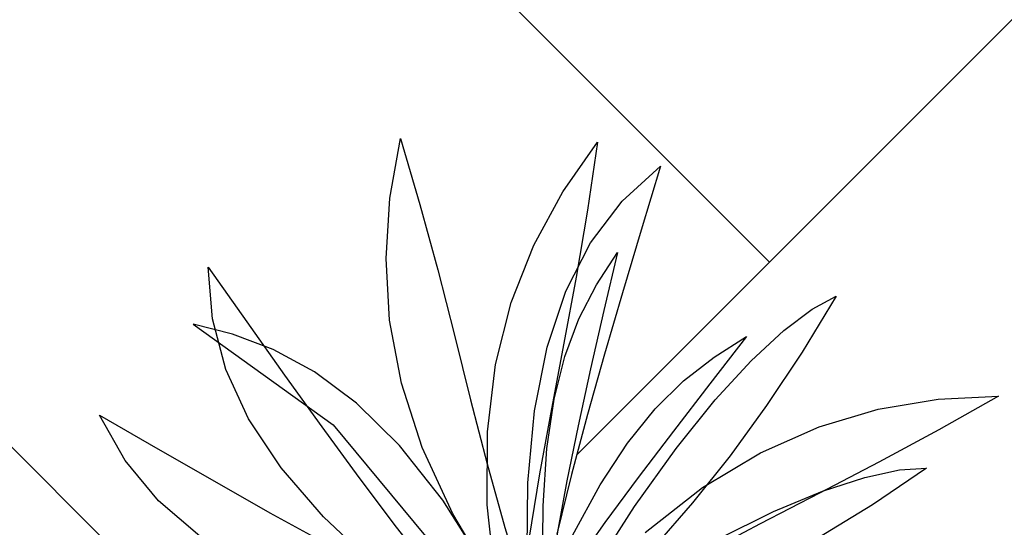
# Model space of a CAD drawing. Units: inches. Extents: x 3590 to 5167, y 65 to 1917.
# Tile 41 of 100: x 5035 to 5065, y 1357 to 1372. Entities that reach past the tile are written whole.
import ezdxf

# ---------------------------------------------------------------- set-up
doc = ezdxf.new("R2010")
doc.units = ezdxf.units.IN
doc.layers.add('A-FLOR-PATT', color=8, linetype='Continuous', lineweight=13)
doc.layers.add('L-PLNT', color=94, linetype='Continuous', lineweight=18)
doc.layers.add('DIENHOA', color=3, linetype='Continuous')

# ---------------------------------------------------------------- blocks, each defined once
blk = doc.blocks.new('Cay03_mb')
at = {"layer": 'DIENHOA'}
for p, q in [((118.6, 555.3), (166.2, 599.1)), ((166.2, 599.1), (142.2, 519.4)), ((79.5, 503.7), (118.6, 555.3)), ((142.2, 519.4), (119, 441.7)), ((48.6, 443.6), (79.5, 503.7)), ((25.5, 374.3), (48.6, 443.6)), ((119, 441.7), (96.7, 365.6)), ((-365.2, 390.3), (-414.4, 402.8)), ((-414.4, 402.8), (-240.2, 277.8)), ((-314.9, 371.3), (-365.2, 390.3)), ((-263.5, 343.5), (-314.9, 371.3)), ((9.9, 295.3), (25.5, 374.3)), ((96.7, 365.6), (75.6, 290.6)), ((-211.2, 304.6), (-263.5, 343.5)), ((436.8, 297.2), (511, 309.6)), ((511, 309.6), (585.9, 313.5)), ((585.9, 313.5), (511.8, 271.4)), ((-158, 252.3), (-211.2, 304.6)), ((1.6, 205.7), (9.9, 295.3)), ((363.4, 275.4), (436.8, 297.2)), ((75.6, 290.6), (55.7, 216.3)), ((-240.2, 277.8), (-88.4, 94.9)), ((290.6, 243.2), (363.4, 275.4)), ((511.8, 271.4), (437.6, 231.5)), ((-104.2, 184.4), (-158, 252.3)), ((218.5, 199.8), (290.6, 243.2)), ((437.6, 231.5), (363.7, 192.9)), ((55.7, 216.3), (37.3, 142.1)), ((0.2, 104.9), (1.6, 205.7)), ((147, 144.1), (218.5, 199.8)), ((-49.6, 98.5), (-104.2, 184.4)), ((363.7, 192.9), (290.2, 154.9)), ((290.2, 154.9), (217.4, 116.6))]:
    blk.add_line(p, q, dxfattribs=at)
for points in [[(23.7, -5.4), (-41, 82.2), (-91.8, 167.1), (-129.7, 249.5), (-155.6, 329.6), (-170.2, 407.8), (-174.7, 484.2), (-169.8, 559.3), (-156.5, 633.1)], [(-156.5, 633.1), (-132.5, 551.3), (-110.5, 470), (-89.8, 389.2), (-69.6, 309), (-49, 229.4), (-27.1, 150.4), (-3.2, 72.1), (23.7, -5.4)], [(-16.4, -26.7), (-38.3, 80), (-48.9, 178.3), (-48.7, 269), (-38.5, 352.6), (-19.1, 429.7), (9, 501), (44.9, 567.1), (87.9, 628.5)], [(87.9, 628.5), (75.5, 544.2), (61.3, 461.2), (46.1, 379.1), (30.8, 297.8), (16.1, 216.9), (2.9, 136), (-8.3, 54.9), (-16.4, -26.7)], [(23.7, -5.4), (19.8, 93), (20.3, 177), (25, 248.5), (34, 309.8), (47.3, 362.7), (64.9, 409.3), (86.8, 451.7), (112.9, 491.9)], [(112.9, 491.9), (96, 419.7), (79.5, 347.4), (63.9, 276.5), (50, 208.4), (38.4, 144.8), (29.7, 86.9), (24.6, 36.3), (23.7, -5.4)], [(-395.6, 473.7), (-347.5, 405.6), (-300.6, 339.5), (-254.3, 275.1), (-208.3, 212.3), (-161.9, 150.9), (-114.8, 90.7), (-66.5, 31.6), (-16.4, -26.7)], [(-16.4, -26.7), (-108.3, 38.6), (-186.9, 101.7), (-252.4, 163.5), (-305.1, 224.4), (-345.4, 285.2), (-373.7, 346.6), (-390.4, 409.2), (-395.6, 473.7)], [(384.3, 437.5), (342.2, 367.8), (298.1, 301.7), (252.6, 239.4), (206.1, 181.1), (159.4, 127.2), (113, 78), (67.6, 33.6), (23.7, -5.4)], [(23.7, -5.4), (79.9, 91.7), (134.1, 176.2), (185.8, 248.4), (234.3, 308.7), (279, 357.3), (319.3, 394.8), (354.6, 421.4), (384.3, 437.5)], [(273.2, 387.3), (227.6, 328.8), (182.3, 270.1), (138.4, 212.3), (97.2, 156.4), (60, 103.4), (27.8, 54.6), (1.9, 10.8), (-16.4, -26.7)], [(-16.4, -26.7), (21.4, 64.2), (57, 140.3), (91.4, 203.3), (125.2, 255.1), (159.5, 297.5), (195, 332.5), (232.7, 361.8), (273.2, 387.3)], [(-530.5, 289.7), (-458.3, 248.1), (-387.9, 207.8), (-318.9, 168.7), (-250.8, 131.1), (-182.9, 94.8), (-114.9, 59.9), (-46.2, 26.5), (23.7, -5.4)], [(23.7, -5.4), (-87.2, 15.2), (-185, 39.6), (-270.3, 68.2), (-343.7, 101.4), (-405.9, 139.7), (-457.3, 183.5), (-498.7, 233.4), (-530.5, 289.7)], [(496.7, 224), (429.4, 178.4), (361.6, 136.9), (294.1, 99.5), (227.5, 66.1), (162.4, 36.7), (99.7, 11.5), (39.8, -9.7), (-16.4, -26.7)], [(-16.4, -26.7), (75.4, 37.9), (160.1, 91.8), (237.3, 135.7), (306.6, 170), (367.6, 195.4), (419.9, 212.5), (463.1, 221.9), (496.7, 224)]]:
    blk.add_lwpolyline(points, dxfattribs=at)

msp = doc.modelspace()

# ---------------------------------------------------------------- hatches: boundary and pattern name
at = {"layer": 'A-FLOR-PATT', "transparency": 33554687}
h = msp.add_hatch(dxfattribs=at)
h.set_pattern_fill('AR-HBONE', color=256, scale=0.2)
h.set_pattern_definition([(45, (-588.972, 0), (0, 28.73682), [60.96, -20.32]), (135, (-574.604, 14.368), (3e-15, 28.73682), [60.96, -20.32])])
h.paths.add_polyline_path([(5071.274, 1796.999), (4933.274, 1796.999), (4933.274, 1753.999), (4962.774, 1753.999, -0.414214), (4928.774, 1719.999), (4933.274, 1718.999), (4933.274, 1334.999), (5071.274, 1334.999)])
h.paths.add_polyline_path([(4951.78, 1521.077), (4951.715, 1521.04), (4951.563, 1520.895)], flags=16)
h.paths.add_polyline_path([(4952.267, 1521.376), (4952.198, 1521.371), (4952.198, 1521.356)], flags=0)
h.paths.add_polyline_path([(4967.051, 1529.728), (4965.231, 1528.694), (4963.411, 1527.714), (4961.756, 1526.851), (4963.589, 1527.449), (4964.036, 1527.478), (4962.975, 1527.249), (4961.76, 1526.852), (4959.792, 1525.834), (4958.005, 1524.895), (4956.24, 1523.93), (4954.504, 1522.919), (4954.129, 1522.682), (4953.361, 1521.997), (4953.366, 1521.998), (4953.605, 1522.064), (4955.106, 1522.761), (4956.921, 1523.434), (4958.678, 1523.915), (4960.358, 1524.2), (4961.945, 1524.286), (4964.171, 1524.108), (4965.958, 1523.309), (4963.863, 1522.976), (4965.187, 1522.499), (4963.366, 1522.497), (4961.545, 1522.487), (4959.764, 1522.461), (4958.304, 1522.419), (4957.974, 1522.388), (4956.307, 1522.232), (4954.718, 1522.071), (4953.251, 1521.899), (4953.525, 1521.623), (4954.331, 1521.379), (4956.243, 1521.23), (4958.039, 1520.93), (4959.684, 1520.483), (4961.16, 1519.896), (4963.107, 1518.8), (4964.393, 1517.325), (4962.973, 1517.726), (4964.558, 1516.661), (4965.407, 1515.708), (4963.507, 1516.322), (4961.68, 1517.005), (4959.935, 1517.745), (4958.282, 1518.528), (4956.732, 1519.343), (4955.295, 1520.175), (4954.672, 1520.572), (4954.513, 1520.627), (4955.658, 1519.318), (4956.703, 1517.982), (4957.644, 1516.647), (4958.485, 1515.334), (4959.55, 1513.524), (4960.438, 1511.769), (4958.841, 1513.62), (4957.452, 1515.325), (4955.819, 1517.459), (4956.665, 1515.448), (4957.111, 1513.923), (4957.447, 1511.714), (4957.076, 1509.793), (4956.538, 1511.11), (4955.992, 1512.569), (4955.444, 1514.125), (4954.898, 1515.735), (4954.357, 1517.356), (4953.824, 1518.943), (4953.305, 1520.452), (4953.065, 1521.116), (4952.971, 1521.146), (4952.949, 1521.086), (4952.73, 1520.199), (4953.37, 1518.024), (4953.757, 1516.373), (4954.051, 1514.765), (4954.264, 1513.221), (4954.471, 1511.131), (4954.497, 1510.402), (4954.409, 1511.76), (4954.264, 1513.221), (4954.051, 1514.765), (4953.757, 1516.373), (4953.37, 1518.024), (4952.877, 1519.698), (4952.716, 1520.141), (4952.533, 1519.059), (4952.374, 1517.789), (4952.219, 1516.312), (4952.046, 1514.6), (4951.833, 1512.626), (4951.557, 1510.363), (4951.203, 1512.168), (4950.852, 1514.339), (4950.985, 1516.376), (4951.66, 1518.286), (4952.593, 1520.481), (4952.357, 1521.13), (4951.855, 1520.328), (4950.839, 1518.908), (4949.777, 1517.587), (4948.916, 1516.617), (4948.111, 1515.256), (4947.089, 1513.554), (4945.889, 1511.615), (4946.326, 1513.402), (4946.562, 1514.249), (4945.528, 1513.327), (4944.581, 1512.531), (4946.018, 1514.508), (4947.204, 1516.048), (4947.893, 1517.313), (4949.307, 1518.764), (4950.414, 1519.767), (4950.451, 1519.806), (4952.267, 1521.376), (4951.645, 1521.493), (4950.404, 1521.18), (4948.044, 1520.359), (4946.119, 1519.452), (4944.572, 1518.475), (4943.35, 1517.443), (4941.997, 1515.92), (4941.661, 1515.275), (4942.813, 1516.99), (4944.572, 1518.475), (4946.119, 1519.452), (4948.044, 1520.359), (4950.404, 1521.18), (4951.645, 1521.493), (4949.647, 1521.868), (4948.6, 1521.756), (4947.126, 1521.57), (4945.42, 1521.348), (4943.45, 1521.105), (4941.183, 1520.856), (4942.86, 1521.613), (4943.873, 1522.03), (4942.952, 1521.909), (4941.41, 1521.485), (4939.543, 1520.67), (4938.968, 1520.226), (4940.733, 1521.299), (4942.952, 1521.909), (4943.702, 1522.008), (4945.894, 1522.7), (4947.565, 1522.714), (4948.921, 1522.566), (4951.131, 1522.183), (4950.971, 1522.297), (4948.129, 1523.006), (4946.035, 1523.707), (4944.232, 1524.521), (4942.707, 1525.461), (4941.444, 1526.537), (4940.43, 1527.761), (4939.649, 1529.143), (4941.421, 1528.122), (4943.147, 1527.132), (4944.841, 1526.175), (4946.514, 1525.25), (4948.179, 1524.359), (4948.365, 1524.263), (4946.475, 1526.045), (4945.181, 1527.54), (4944.19, 1529.033), (4943.496, 1530.54), (4943.278, 1531.36), (4942.498, 1531.919), (4943.114, 1531.762), (4942.959, 1533.659), (4944.14, 1531.989), (4944.612, 1531.323), (4946.202, 1530.463), (4947.486, 1529.509), (4948.79, 1528.226), (4950.368, 1526.237), (4949.485, 1528.155), (4948.851, 1530.123), (4948.491, 1532.041), (4948.381, 1533.918), (4948.501, 1535.76), (4948.827, 1537.573), (4949.418, 1535.565), (4949.957, 1533.569), (4950.464, 1531.586), (4950.961, 1529.617), (4951.391, 1527.954), (4951.724, 1530.687), (4952.201, 1532.58), (4952.889, 1534.33), (4953.77, 1535.951), (4954.827, 1537.46), (4954.521, 1535.39), (4954.273, 1533.937), (4955.58, 1535.663), (4956.748, 1536.739), (4956.159, 1534.78), (4955.589, 1532.873), (4955.043, 1531.006), (4954.525, 1529.166), (4954.038, 1527.341), (4953.638, 1525.733), (4953.611, 1525.586), (4953.398, 1524.166), (4953.382, 1524.009), (4954.07, 1525.476), (4954.912, 1527.022), (4956.136, 1528.894), (4957.847, 1530.577), (4959.376, 1531.54), (4958.256, 1530.104), (4957.143, 1528.663), (4956.066, 1527.243), (4955.056, 1525.871), (4954.141, 1524.571), (4953.352, 1523.372), (4953.311, 1523.303), (4953.273, 1522.925), (4953.261, 1522.382), (4954.103, 1523.373), (4954.63, 1524.284), (4955.961, 1526.358), (4957.23, 1528.13), (4958.421, 1529.609), (4960.037, 1531.368), (4961.374, 1532.375), (4962.101, 1532.77), (4961.07, 1531.061), (4959.987, 1529.438), (4958.869, 1527.908), (4958.15, 1527.007), (4959.803, 1528.003), (4961.589, 1528.793), (4963.391, 1529.328), (4965.211, 1529.632)], flags=16)
h.paths.add_polyline_path([(4962.944, 1523.182), (4961.107, 1523.422), (4960.392, 1523.362), (4962.35, 1523.331)], flags=0)
h.paths.add_polyline_path([(5049.541, 1584.551), (5049.476, 1584.515), (5049.325, 1584.37)], flags=16)
h.paths.add_polyline_path([(5050.028, 1584.851), (5049.959, 1584.845), (5049.959, 1584.83)], flags=0)
h.paths.add_polyline_path([(5042.333, 1581.949), (5043.88, 1582.926), (5045.806, 1583.833), (5048.165, 1584.654), (5049.406, 1584.967), (5047.408, 1585.342), (5046.361, 1585.231), (5044.888, 1585.044), (5043.181, 1584.822), (5041.211, 1584.579), (5038.944, 1584.33), (5040.622, 1585.087), (5041.634, 1585.504), (5040.713, 1585.383), (5039.171, 1584.959), (5037.304, 1584.144), (5036.729, 1583.7), (5038.494, 1584.773), (5040.713, 1585.383), (5041.463, 1585.482), (5043.655, 1586.174), (5045.326, 1586.188), (5046.682, 1586.04), (5048.893, 1585.657), (5048.732, 1585.771), (5045.891, 1586.48), (5043.796, 1587.181), (5041.994, 1587.996), (5040.468, 1588.935), (5039.205, 1590.011), (5038.191, 1591.235), (5037.41, 1592.617), (5039.182, 1591.596), (5040.909, 1590.607), (5042.602, 1589.649), (5044.275, 1588.724), (5045.94, 1587.833), (5046.126, 1587.738), (5044.237, 1589.519), (5042.942, 1591.015), (5041.952, 1592.508), (5041.257, 1594.014), (5041.039, 1594.834), (5040.26, 1595.393), (5040.875, 1595.237), (5040.721, 1597.133), (5041.901, 1595.463), (5042.373, 1594.798), (5043.963, 1593.938), (5045.247, 1592.983), (5046.552, 1591.701), (5048.129, 1589.712), (5047.247, 1591.63), (5046.613, 1593.597), (5046.252, 1595.515), (5046.142, 1597.392), (5046.262, 1599.234), (5046.588, 1601.047), (5047.179, 1599.039), (5047.718, 1597.043), (5048.225, 1595.06), (5048.722, 1593.091), (5049.152, 1591.429), (5049.485, 1594.161), (5049.962, 1596.054), (5050.65, 1597.804), (5051.532, 1599.425), (5052.589, 1600.934), (5052.283, 1598.864), (5052.034, 1597.411), (5053.341, 1599.137), (5054.509, 1600.213), (5053.92, 1598.254), (5053.35, 1596.348), (5052.805, 1594.48), (5052.286, 1592.64), (5051.799, 1590.815), (5051.4, 1589.207), (5051.373, 1589.06), (5051.159, 1587.64), (5051.143, 1587.483), (5051.831, 1588.95), (5052.673, 1590.496), (5053.898, 1592.368), (5055.608, 1594.051), (5057.137, 1595.014), (5056.017, 1593.578), (5054.904, 1592.137), (5053.828, 1590.717), (5052.817, 1589.345), (5051.902, 1588.046), (5051.113, 1586.846), (5051.072, 1586.777), (5051.034, 1586.399), (5051.022, 1585.856), (5051.864, 1586.847), (5052.391, 1587.758), (5053.723, 1589.832), (5054.991, 1591.604), (5056.182, 1593.083), (5057.798, 1594.842), (5059.135, 1595.849), (5059.863, 1596.244), (5058.831, 1594.535), (5057.749, 1592.912), (5056.63, 1591.382), (5055.912, 1590.482), (5057.564, 1591.477), (5059.35, 1592.267), (5061.152, 1592.802), (5062.972, 1593.106), (5064.812, 1593.203), (5062.992, 1592.169), (5061.172, 1591.188), (5059.518, 1590.325), (5061.35, 1590.924), (5061.797, 1590.952), (5060.737, 1590.723), (5059.521, 1590.326), (5057.553, 1589.308), (5055.766, 1588.369), (5054.002, 1587.404), (5052.265, 1586.393), (5051.891, 1586.156), (5051.122, 1585.471), (5051.127, 1585.472), (5051.366, 1585.538), (5052.867, 1586.235), (5054.682, 1586.908), (5056.439, 1587.389), (5058.12, 1587.675), (5059.706, 1587.76), (5061.933, 1587.583), (5063.719, 1586.783), (5061.624, 1586.45), (5062.949, 1585.973), (5061.127, 1585.971), (5059.307, 1585.961), (5057.525, 1585.935), (5056.065, 1585.893), (5055.735, 1585.862), (5054.068, 1585.707), (5052.479, 1585.546), (5051.012, 1585.373), (5051.286, 1585.097), (5052.092, 1584.853), (5054.004, 1584.704), (5055.8, 1584.404), (5057.446, 1583.958), (5058.921, 1583.37), (5060.868, 1582.274), (5062.154, 1580.799), (5060.734, 1581.2), (5062.32, 1580.135), (5063.168, 1579.182), (5061.269, 1579.796), (5059.441, 1580.479), (5057.696, 1581.219), (5056.043, 1582.003), (5054.493, 1582.817), (5053.057, 1583.649), (5052.433, 1584.047), (5052.274, 1584.101), (5053.42, 1582.793), (5054.464, 1581.457), (5055.405, 1580.121), (5056.247, 1578.809), (5057.311, 1576.998), (5058.199, 1575.244), (5056.602, 1577.094), (5055.213, 1578.799), (5053.58, 1580.933), (5054.427, 1578.922), (5054.872, 1577.397), (5055.208, 1575.189), (5054.838, 1573.267), (5054.299, 1574.584), (5053.754, 1576.043), (5053.206, 1577.599), (5052.659, 1579.209), (5052.118, 1580.83), (5051.585, 1582.417), (5051.066, 1583.927), (5050.826, 1584.59), (5050.733, 1584.62), (5050.711, 1584.561), (5050.491, 1583.673), (5051.131, 1581.498), (5051.518, 1579.847), (5051.813, 1578.24), (5052.026, 1576.695), (5052.233, 1574.605), (5052.258, 1573.876), (5052.17, 1575.234), (5052.026, 1576.695), (5051.813, 1578.24), (5051.518, 1579.847), (5051.131, 1581.498), (5050.638, 1583.172), (5050.477, 1583.615), (5050.294, 1582.533), (5050.136, 1581.263), (5049.981, 1579.786), (5049.807, 1578.074), (5049.594, 1576.1), (5049.318, 1573.837), (5048.965, 1575.642), (5048.613, 1577.813), (5048.747, 1579.85), (5049.421, 1581.76), (5050.354, 1583.955), (5050.118, 1584.604), (5049.616, 1583.802), (5048.6, 1582.382), (5047.538, 1581.061), (5046.677, 1580.091), (5045.872, 1578.73), (5044.85, 1577.028), (5043.651, 1575.089), (5044.087, 1576.877), (5044.324, 1577.723), (5043.289, 1576.801), (5042.342, 1576.005), (5043.779, 1577.982), (5044.966, 1579.522), (5045.655, 1580.787), (5047.068, 1582.239), (5048.175, 1583.241), (5048.213, 1583.28), (5050.028, 1584.851), (5049.406, 1584.967), (5048.165, 1584.654), (5045.806, 1583.833), (5043.88, 1582.926), (5042.333, 1581.949), (5041.111, 1580.917), (5039.758, 1579.394), (5039.423, 1578.749), (5040.575, 1580.464)], flags=16)
h.paths.add_polyline_path([(4954.799, 1533.12), (4954.262, 1532.079), (4953.831, 1530.935), (4953.505, 1529.636), (4953.283, 1528.133), (4953.167, 1526.376), (4953.156, 1524.315), (4953.277, 1521.236), (4952.802, 1521.842), (4951.557, 1521.998), (4950.976, 1521.961), (4952.661, 1521.941), (4952.802, 1521.842), (4953.152, 1523.593), (4953.167, 1526.376), (4953.283, 1528.133), (4953.609, 1530.346), (4954.456, 1532.592)], flags=0)
h.paths.add_polyline_path([(5050.563, 1585.316), (5049.318, 1585.472), (5048.737, 1585.435), (5050.422, 1585.415), (5050.563, 1585.316), (5050.914, 1587.067), (5050.928, 1589.851), (5051.045, 1591.607), (5051.371, 1593.82), (5052.217, 1596.066), (5052.56, 1596.594), (5052.024, 1595.554), (5051.592, 1594.409), (5051.266, 1593.11), (5051.045, 1591.607), (5050.928, 1589.851), (5050.918, 1587.789), (5051.038, 1584.71)], flags=0)
h.paths.add_polyline_path([(5058.153, 1586.836), (5060.111, 1586.805), (5060.705, 1586.656), (5058.868, 1586.896)], flags=0)
h.paths.add_polyline_path([(5049.541, 1430.936), (5049.476, 1430.9), (5049.325, 1430.755)], flags=16)
h.paths.add_polyline_path([(5050.028, 1431.236), (5049.959, 1431.231), (5049.959, 1431.215)], flags=0)
h.paths.add_polyline_path([(5046.588, 1447.432), (5047.179, 1445.425), (5047.718, 1443.429), (5048.225, 1441.446), (5048.722, 1439.476), (5049.152, 1437.814), (5049.485, 1440.546), (5049.962, 1442.439), (5050.65, 1444.189), (5051.532, 1445.811), (5052.589, 1447.319), (5052.283, 1445.249), (5052.034, 1443.796), (5053.341, 1445.522), (5054.509, 1446.598), (5053.92, 1444.64), (5053.35, 1442.733), (5052.805, 1440.865), (5052.286, 1439.025), (5051.799, 1437.201), (5051.4, 1435.592), (5051.373, 1435.445), (5051.159, 1434.025), (5051.143, 1433.868), (5051.831, 1435.335), (5052.673, 1436.881), (5053.898, 1438.753), (5055.608, 1440.436), (5057.137, 1441.4), (5056.017, 1439.963), (5054.904, 1438.522), (5053.828, 1437.102), (5052.817, 1435.73), (5051.902, 1434.431), (5051.113, 1433.231), (5051.072, 1433.162), (5051.034, 1432.784), (5051.022, 1432.242), (5051.864, 1433.232), (5052.391, 1434.143), (5053.723, 1436.217), (5054.991, 1437.989), (5056.182, 1439.468), (5057.798, 1441.227), (5059.135, 1442.235), (5059.863, 1442.629), (5058.831, 1440.921), (5057.749, 1439.298), (5056.63, 1437.767), (5055.912, 1436.867), (5057.564, 1437.863), (5059.35, 1438.652), (5061.152, 1439.187), (5062.972, 1439.491), (5064.812, 1439.588), (5062.992, 1438.554), (5061.172, 1437.573), (5059.518, 1436.71), (5061.35, 1437.309), (5061.797, 1437.337), (5060.737, 1437.108), (5059.521, 1436.711), (5057.553, 1435.693), (5055.766, 1434.754), (5054.002, 1433.789), (5052.265, 1432.778), (5051.891, 1432.541), (5051.122, 1431.856), (5051.127, 1431.857), (5051.366, 1431.923), (5052.867, 1432.62), (5054.682, 1433.293), (5056.439, 1433.775), (5058.12, 1434.06), (5059.706, 1434.145), (5061.933, 1433.968), (5063.719, 1433.168), (5061.624, 1432.835), (5062.949, 1432.358), (5061.127, 1432.357), (5059.307, 1432.346), (5057.525, 1432.32), (5056.065, 1432.278), (5055.735, 1432.248), (5054.068, 1432.092), (5052.479, 1431.931), (5051.012, 1431.759), (5051.286, 1431.482), (5052.092, 1431.238), (5054.004, 1431.089), (5055.8, 1430.789), (5057.446, 1430.343), (5058.921, 1429.755), (5060.868, 1428.66), (5062.154, 1427.185), (5060.734, 1427.585), (5062.32, 1426.52), (5063.168, 1425.567), (5061.269, 1426.181), (5059.441, 1426.865), (5057.696, 1427.604), (5056.043, 1428.388), (5054.493, 1429.202), (5053.057, 1430.034), (5052.433, 1430.432), (5052.274, 1430.487), (5053.42, 1429.178), (5054.464, 1427.842), (5055.405, 1426.506), (5056.247, 1425.194), (5057.311, 1423.383), (5058.199, 1421.629), (5056.602, 1423.479), (5055.213, 1425.184), (5053.58, 1427.318), (5054.427, 1425.307), (5054.872, 1423.782), (5055.208, 1421.574), (5054.838, 1419.652), (5054.299, 1420.97), (5053.754, 1422.428), (5053.206, 1423.984), (5052.659, 1425.595), (5052.118, 1427.215), (5051.585, 1428.802), (5051.066, 1430.312), (5050.826, 1430.975), (5050.733, 1431.005), (5050.711, 1430.946), (5050.491, 1430.058), (5051.131, 1427.883), (5051.518, 1426.232), (5051.813, 1424.625), (5052.026, 1423.081), (5052.233, 1420.991), (5052.258, 1420.261), (5052.17, 1421.619), (5052.026, 1423.081), (5051.813, 1424.625), (5051.518, 1426.232), (5051.131, 1427.883), (5050.638, 1429.558), (5050.477, 1430.001), (5050.294, 1428.918), (5050.136, 1427.648), (5049.981, 1426.171), (5049.807, 1424.459), (5049.594, 1422.485), (5049.318, 1420.222), (5048.965, 1422.028), (5048.613, 1424.199), (5048.747, 1426.235), (5049.421, 1428.146), (5050.354, 1430.34), (5050.118, 1430.989), (5049.616, 1430.187), (5048.6, 1428.768), (5047.538, 1427.446), (5046.677, 1426.477), (5045.872, 1425.116), (5044.85, 1423.413), (5043.651, 1421.474), (5044.087, 1423.262), (5044.324, 1424.109), (5043.289, 1423.186), (5042.342, 1422.391), (5043.779, 1424.368), (5044.966, 1425.907), (5045.655, 1427.173), (5047.068, 1428.624), (5048.175, 1429.627), (5048.213, 1429.666), (5050.028, 1431.236), (5049.406, 1431.353), (5048.165, 1431.039), (5045.806, 1430.218), (5043.88, 1429.311), (5042.333, 1428.334), (5041.111, 1427.302), (5039.758, 1425.779), (5039.423, 1425.134), (5040.575, 1426.849), (5042.333, 1428.334), (5043.88, 1429.311), (5045.806, 1430.218), (5048.165, 1431.039), (5049.406, 1431.353), (5047.408, 1431.727), (5046.361, 1431.616), (5044.888, 1431.429), (5043.181, 1431.207), (5041.211, 1430.964), (5038.944, 1430.715), (5040.622, 1431.472), (5041.634, 1431.89), (5040.713, 1431.769), (5039.171, 1431.345), (5037.304, 1430.53), (5036.729, 1430.085), (5038.494, 1431.158), (5040.713, 1431.769), (5041.463, 1431.867), (5043.655, 1432.559), (5045.326, 1432.573), (5046.682, 1432.425), (5048.893, 1432.042), (5048.732, 1432.156), (5045.891, 1432.865), (5043.796, 1433.566), (5041.994, 1434.381), (5040.468, 1435.321), (5039.205, 1436.396), (5038.191, 1437.62), (5037.41, 1439.002), (5039.182, 1437.982), (5040.909, 1436.992), (5042.602, 1436.034), (5044.275, 1435.109), (5045.94, 1434.218), (5046.126, 1434.123), (5044.237, 1435.904), (5042.942, 1437.4), (5041.952, 1438.893), (5041.257, 1440.399), (5041.039, 1441.219), (5040.26, 1441.778), (5040.875, 1441.622), (5040.721, 1443.518), (5041.901, 1441.848), (5042.373, 1441.183), (5043.963, 1440.323), (5045.247, 1439.369), (5046.552, 1438.086), (5048.129, 1436.097), (5047.247, 1438.015), (5046.613, 1439.982), (5046.252, 1441.901), (5046.142, 1443.778), (5046.262, 1445.619)], flags=16)
h.paths.add_polyline_path([(5052.382, 1444.255), (5051.623, 1442.78), (5052.024, 1441.939), (5052.56, 1442.98)], flags=0)
h.paths.add_polyline_path([(5050.563, 1431.701), (5049.318, 1431.857), (5048.737, 1431.821), (5050.422, 1431.8)], flags=0)
h.paths.add_polyline_path([(5058.153, 1433.221), (5060.111, 1433.19), (5060.705, 1433.041), (5058.868, 1433.281)], flags=0)
h.paths.add_polyline_path([(5049.541, 1352.285), (5049.476, 1352.249), (5049.325, 1352.104)], flags=16)
h.paths.add_polyline_path([(5050.028, 1352.585), (5049.959, 1352.58), (5049.959, 1352.564)], flags=0)
h.paths.add_polyline_path([(5046.588, 1368.781), (5047.179, 1366.774), (5047.718, 1364.778), (5048.225, 1362.795), (5048.722, 1360.825), (5049.152, 1359.163), (5049.485, 1361.896), (5049.962, 1363.789), (5050.65, 1365.538), (5051.532, 1367.16), (5052.589, 1368.669), (5052.283, 1366.598), (5052.034, 1365.145), (5053.341, 1366.871), (5054.509, 1367.947), (5053.92, 1365.989), (5053.35, 1364.082), (5052.805, 1362.214), (5052.286, 1360.374), (5051.799, 1358.55), (5051.4, 1356.942), (5051.373, 1356.794), (5051.159, 1355.374), (5051.143, 1355.218), (5051.831, 1356.684), (5052.673, 1358.23), (5053.898, 1360.102), (5055.608, 1361.786), (5057.137, 1362.749), (5056.017, 1361.313), (5054.904, 1359.872), (5053.828, 1358.452), (5052.817, 1357.079), (5051.902, 1355.78), (5051.113, 1354.581), (5051.072, 1354.512), (5051.034, 1354.133), (5051.022, 1353.591), (5051.864, 1354.581), (5052.391, 1355.492), (5053.723, 1357.566), (5054.991, 1359.338), (5056.182, 1360.817), (5057.798, 1362.577), (5059.135, 1363.584), (5059.863, 1363.979), (5058.831, 1362.27), (5057.749, 1360.647), (5056.63, 1359.117), (5055.912, 1358.216), (5057.564, 1359.212), (5059.35, 1360.001), (5061.152, 1360.536), (5062.972, 1360.841), (5064.812, 1360.937), (5062.992, 1359.903), (5061.172, 1358.923), (5059.518, 1358.059), (5061.35, 1358.658), (5061.797, 1358.687), (5060.737, 1358.458), (5059.521, 1358.061), (5057.553, 1357.043), (5055.766, 1356.103), (5054.002, 1355.138), (5052.265, 1354.127), (5051.891, 1353.89), (5051.122, 1353.206), (5051.127, 1353.206), (5051.366, 1353.272), (5052.867, 1353.969), (5054.682, 1354.643), (5056.439, 1355.124), (5058.12, 1355.409), (5059.706, 1355.495), (5061.933, 1355.317), (5063.719, 1354.518), (5061.624, 1354.184), (5062.949, 1353.708), (5061.127, 1353.706), (5059.307, 1353.695), (5057.525, 1353.669), (5056.065, 1353.627), (5055.735, 1353.597), (5054.068, 1353.441), (5052.479, 1353.28), (5051.012, 1353.108), (5051.286, 1352.831), (5052.092, 1352.587), (5054.004, 1352.439), (5055.8, 1352.138), (5057.446, 1351.692), (5058.921, 1351.104), (5060.868, 1350.009), (5062.154, 1348.534), (5060.734, 1348.935), (5062.32, 1347.869), (5063.168, 1346.916), (5061.269, 1347.53), (5059.441, 1348.214), (5057.696, 1348.954), (5056.043, 1349.737), (5054.493, 1350.551), (5053.057, 1351.383), (5052.433, 1351.781), (5052.274, 1351.836), (5053.42, 1350.527), (5054.464, 1349.191), (5055.405, 1347.855), (5056.247, 1346.543), (5057.311, 1344.733), (5058.199, 1342.978), (5056.602, 1344.828), (5055.213, 1346.534), (5053.58, 1348.667), (5054.427, 1346.656), (5054.872, 1345.132), (5055.208, 1342.923), (5054.838, 1341.002), (5054.299, 1342.319), (5053.754, 1343.778), (5053.206, 1345.334), (5052.659, 1346.944), (5052.118, 1348.564), (5051.585, 1350.151), (5051.066, 1351.661), (5050.826, 1352.324), (5050.733, 1352.355), (5050.711, 1352.295), (5050.491, 1351.408), (5051.131, 1349.232), (5051.518, 1347.581), (5051.813, 1345.974), (5052.026, 1344.43), (5052.233, 1342.34), (5052.258, 1341.61), (5052.17, 1342.969), (5052.026, 1344.43), (5051.813, 1345.974), (5051.518, 1347.581), (5051.131, 1349.232), (5050.638, 1350.907), (5050.477, 1351.35), (5050.294, 1350.267), (5050.136, 1348.997), (5049.981, 1347.52), (5049.807, 1345.809), (5049.594, 1343.835), (5049.318, 1341.571), (5048.965, 1343.377), (5048.613, 1345.548), (5048.747, 1347.585), (5049.421, 1349.495), (5050.354, 1351.689), (5050.118, 1352.339), (5049.616, 1351.536), (5048.6, 1350.117), (5047.538, 1348.795), (5046.677, 1347.826), (5045.872, 1346.465), (5044.85, 1344.763), (5043.651, 1342.824), (5044.087, 1344.611), (5044.324, 1345.458), (5043.289, 1344.535), (5042.342, 1343.74), (5043.779, 1345.717), (5044.966, 1347.256), (5045.655, 1348.522), (5047.068, 1349.973), (5048.175, 1350.976), (5048.213, 1351.015), (5050.028, 1352.585), (5049.406, 1352.702), (5048.165, 1352.388), (5045.806, 1351.567), (5043.88, 1350.661), (5042.333, 1349.683), (5041.111, 1348.651), (5039.758, 1347.128), (5039.423, 1346.483), (5040.575, 1348.198), (5042.333, 1349.683), (5043.88, 1350.661), (5045.806, 1351.567), (5048.165, 1352.388), (5049.406, 1352.702), (5047.408, 1353.076), (5046.361, 1352.965), (5044.888, 1352.779), (5043.181, 1352.556), (5041.211, 1352.313), (5038.944, 1352.065), (5040.622, 1352.821), (5041.634, 1353.239), (5040.713, 1353.118), (5039.171, 1352.694), (5037.304, 1351.879), (5036.729, 1351.434), (5038.494, 1352.508), (5040.713, 1353.118), (5041.463, 1353.216), (5043.655, 1353.909), (5045.326, 1353.923), (5046.682, 1353.774), (5048.893, 1353.391), (5048.732, 1353.506), (5045.891, 1354.214), (5043.796, 1354.915), (5041.994, 1355.73), (5040.468, 1356.67), (5039.205, 1357.746), (5038.191, 1358.969), (5037.41, 1360.352), (5039.182, 1359.331), (5040.909, 1358.341), (5042.602, 1357.383), (5044.275, 1356.458), (5045.94, 1355.567), (5046.126, 1355.472), (5044.237, 1357.253), (5042.942, 1358.749), (5041.952, 1360.242), (5041.257, 1361.748), (5041.039, 1362.568), (5040.26, 1363.128), (5040.875, 1362.971), (5040.721, 1364.867), (5041.901, 1363.197), (5042.373, 1362.532), (5043.963, 1361.672), (5045.247, 1360.718), (5046.552, 1359.435), (5048.129, 1357.446), (5047.247, 1359.364), (5046.613, 1361.331), (5046.252, 1363.25), (5046.142, 1365.127), (5046.262, 1366.969)], flags=16)
h.paths.add_polyline_path([(5052.382, 1365.604), (5051.623, 1364.129), (5052.024, 1363.288), (5052.56, 1364.329)], flags=0)
h.paths.add_polyline_path([(4951.78, 1698.041), (4951.715, 1698.005), (4951.563, 1697.859)], flags=16)
h.paths.add_polyline_path([(4952.267, 1698.341), (4952.198, 1698.335), (4952.198, 1698.32)], flags=0)
h.paths.add_polyline_path([(4957.076, 1686.757), (4956.538, 1688.074), (4955.992, 1689.533), (4955.444, 1691.089), (4954.898, 1692.699), (4954.357, 1694.32), (4953.824, 1695.907), (4953.305, 1697.417), (4953.065, 1698.08), (4952.971, 1698.11), (4952.949, 1698.051), (4952.73, 1697.163), (4953.37, 1694.988), (4953.757, 1693.337), (4954.051, 1691.729), (4954.264, 1690.185), (4954.471, 1688.095), (4954.497, 1687.366), (4954.409, 1688.724), (4954.264, 1690.185), (4954.051, 1691.729), (4953.757, 1693.337), (4953.37, 1694.988), (4952.877, 1696.662), (4952.716, 1697.105), (4952.533, 1696.023), (4952.374, 1694.753), (4952.219, 1693.276), (4952.046, 1691.564), (4951.833, 1689.59), (4951.557, 1687.327), (4951.203, 1689.132), (4950.852, 1691.303), (4950.985, 1693.34), (4951.66, 1695.25), (4952.593, 1697.445), (4952.357, 1698.094), (4951.855, 1697.292), (4950.839, 1695.872), (4949.777, 1694.551), (4948.916, 1693.581), (4948.111, 1692.22), (4947.089, 1690.518), (4945.889, 1688.579), (4946.326, 1690.366), (4946.562, 1691.213), (4945.528, 1690.291), (4944.581, 1689.495), (4946.018, 1691.472), (4947.204, 1693.012), (4947.893, 1694.277), (4949.307, 1695.729), (4950.414, 1696.731), (4950.451, 1696.77), (4952.267, 1698.341), (4951.645, 1698.457), (4950.404, 1698.144), (4948.044, 1697.323), (4946.119, 1696.416), (4944.572, 1695.439), (4943.35, 1694.407), (4941.997, 1692.884), (4941.661, 1692.239), (4942.813, 1693.954), (4944.572, 1695.439), (4946.119, 1696.416), (4948.044, 1697.323), (4950.404, 1698.144), (4951.645, 1698.457), (4949.647, 1698.832), (4948.6, 1698.72), (4947.126, 1698.534), (4945.42, 1698.312), (4943.45, 1698.069), (4941.183, 1697.82), (4942.86, 1698.577), (4943.873, 1698.994), (4942.952, 1698.873), (4941.41, 1698.449), (4939.543, 1697.634), (4938.968, 1697.19), (4940.733, 1698.263), (4942.952, 1698.873), (4943.702, 1698.972), (4945.894, 1699.664), (4947.565, 1699.678), (4948.921, 1699.53), (4951.131, 1699.147), (4950.971, 1699.261), (4948.129, 1699.97), (4946.035, 1700.671), (4944.232, 1701.486), (4942.707, 1702.425), (4941.444, 1703.501), (4940.43, 1704.725), (4939.649, 1706.107), (4941.421, 1705.086), (4943.147, 1704.097), (4944.841, 1703.139), (4946.514, 1702.214), (4948.179, 1701.323), (4948.365, 1701.227), (4946.475, 1703.009), (4945.181, 1704.505), (4944.19, 1705.997), (4943.496, 1707.504), (4943.278, 1708.324), (4942.498, 1708.883), (4943.114, 1708.727), (4942.959, 1710.623), (4944.14, 1708.953), (4944.612, 1708.287), (4946.202, 1707.428), (4947.486, 1706.473), (4948.79, 1705.191), (4950.368, 1703.202), (4949.485, 1705.12), (4948.851, 1707.087), (4948.491, 1709.005), (4948.381, 1710.882), (4948.501, 1712.724), (4948.827, 1714.537), (4949.418, 1712.529), (4949.957, 1710.533), (4950.464, 1708.55), (4950.961, 1706.581), (4951.391, 1704.919), (4951.724, 1707.651), (4952.201, 1709.544), (4952.889, 1711.294), (4953.77, 1712.915), (4954.827, 1714.424), (4954.521, 1712.354), (4954.273, 1710.901), (4955.58, 1712.627), (4956.748, 1713.703), (4956.159, 1711.744), (4955.589, 1709.837), (4955.043, 1707.97), (4954.525, 1706.13), (4954.038, 1704.305), (4953.638, 1702.697), (4953.611, 1702.55), (4953.398, 1701.13), (4953.382, 1700.973), (4954.07, 1702.44), (4954.912, 1703.986), (4956.136, 1705.858), (4957.847, 1707.541), (4959.376, 1708.504), (4958.256, 1707.068), (4957.143, 1705.627), (4956.066, 1704.207), (4955.056, 1702.835), (4954.141, 1701.536), (4953.352, 1700.336), (4953.311, 1700.267), (4953.273, 1699.889), (4953.261, 1699.346), (4954.103, 1700.337), (4954.63, 1701.248), (4955.961, 1703.322), (4957.23, 1705.094), (4958.421, 1706.573), (4960.037, 1708.332), (4961.374, 1709.339), (4962.101, 1709.734), (4961.07, 1708.025), (4959.987, 1706.402), (4958.869, 1704.872), (4958.15, 1703.972), (4959.803, 1704.967), (4961.589, 1705.757), (4963.391, 1706.292), (4965.211, 1706.596), (4967.051, 1706.692), (4965.231, 1705.659), (4963.411, 1704.678), (4961.756, 1703.815), (4963.589, 1704.413), (4964.036, 1704.442), (4962.975, 1704.213), (4961.76, 1703.816), (4959.792, 1702.798), (4958.005, 1701.859), (4956.24, 1700.894), (4954.504, 1699.883), (4954.129, 1699.646), (4953.361, 1698.961), (4953.366, 1698.962), (4953.605, 1699.028), (4955.106, 1699.725), (4956.921, 1700.398), (4958.678, 1700.879), (4960.358, 1701.164), (4961.945, 1701.25), (4964.171, 1701.073), (4965.958, 1700.273), (4963.863, 1699.94), (4965.187, 1699.463), (4963.366, 1699.461), (4961.545, 1699.451), (4959.764, 1699.425), (4958.304, 1699.383), (4957.974, 1699.352), (4956.307, 1699.197), (4954.718, 1699.036), (4953.251, 1698.863), (4953.525, 1698.587), (4954.331, 1698.343), (4956.243, 1698.194), (4958.039, 1697.894), (4959.684, 1697.447), (4961.16, 1696.86), (4963.107, 1695.764), (4964.393, 1694.289), (4962.973, 1694.69), (4964.558, 1693.625), (4965.407, 1692.672), (4963.507, 1693.286), (4961.68, 1693.969), (4959.935, 1694.709), (4958.282, 1695.492), (4956.732, 1696.307), (4955.295, 1697.139), (4954.672, 1697.536), (4954.513, 1697.591), (4955.658, 1696.282), (4956.703, 1694.946), (4957.644, 1693.611), (4958.485, 1692.298), (4959.55, 1690.488), (4960.438, 1688.733), (4958.841, 1690.584), (4957.452, 1692.289), (4955.819, 1694.423), (4956.665, 1692.412), (4957.111, 1690.887), (4957.447, 1688.678)], flags=16)
h.paths.add_polyline_path([(5050.563, 1353.05), (5049.318, 1353.207), (5048.737, 1353.17), (5050.422, 1353.15)], flags=0)
h.paths.add_polyline_path([(4951.78, 1351.486), (4951.715, 1351.45), (4951.563, 1351.305)], flags=16)
h.paths.add_polyline_path([(4952.267, 1351.786), (4952.198, 1351.78), (4952.198, 1351.765)], flags=0)
h.paths.add_polyline_path([(4954.827, 1367.869), (4954.521, 1365.799), (4954.273, 1364.346), (4955.58, 1366.072), (4956.748, 1367.148), (4956.159, 1365.19), (4955.589, 1363.283), (4955.043, 1361.415), (4954.525, 1359.575), (4954.038, 1357.751), (4953.638, 1356.142), (4953.611, 1355.995), (4953.398, 1354.575), (4953.382, 1354.418), (4954.07, 1355.885), (4954.912, 1357.431), (4956.136, 1359.303), (4957.847, 1360.986), (4959.376, 1361.95), (4958.256, 1360.513), (4957.143, 1359.072), (4956.066, 1357.652), (4955.056, 1356.28), (4954.141, 1354.981), (4953.352, 1353.781), (4953.311, 1353.712), (4953.273, 1353.334), (4953.261, 1352.792), (4954.103, 1353.782), (4954.63, 1354.693), (4955.961, 1356.767), (4957.23, 1358.539), (4958.421, 1360.018), (4960.037, 1361.777), (4961.374, 1362.785), (4962.101, 1363.179), (4961.07, 1361.471), (4959.987, 1359.848), (4958.869, 1358.317), (4958.15, 1357.417), (4959.803, 1358.413), (4961.589, 1359.202), (4963.391, 1359.737), (4965.211, 1360.041), (4967.051, 1360.138), (4965.231, 1359.104), (4963.411, 1358.123), (4961.756, 1357.26), (4963.589, 1357.859), (4964.036, 1357.887), (4962.975, 1357.658), (4961.76, 1357.261), (4959.792, 1356.243), (4958.005, 1355.304), (4956.24, 1354.339), (4954.504, 1353.328), (4954.129, 1353.091), (4953.361, 1352.406), (4953.366, 1352.407), (4953.605, 1352.473), (4955.106, 1353.17), (4956.921, 1353.843), (4958.678, 1354.325), (4960.358, 1354.61), (4961.945, 1354.695), (4964.171, 1354.518), (4965.958, 1353.718), (4963.863, 1353.385), (4965.187, 1352.908), (4963.366, 1352.907), (4961.545, 1352.896), (4959.764, 1352.87), (4958.304, 1352.828), (4957.974, 1352.798), (4956.307, 1352.642), (4954.718, 1352.481), (4953.251, 1352.309), (4953.525, 1352.032), (4954.331, 1351.788), (4956.243, 1351.639), (4958.039, 1351.339), (4959.684, 1350.893), (4961.16, 1350.305), (4963.107, 1349.21), (4964.393, 1347.735), (4962.973, 1348.135), (4964.558, 1347.07), (4965.407, 1346.117), (4963.507, 1346.731), (4961.68, 1347.414), (4959.935, 1348.154), (4958.282, 1348.938), (4956.732, 1349.752), (4955.295, 1350.584), (4954.672, 1350.982), (4954.513, 1351.036), (4955.658, 1349.728), (4956.703, 1348.392), (4957.644, 1347.056), (4958.485, 1345.744), (4959.55, 1343.933), (4960.438, 1342.179), (4958.841, 1344.029), (4957.452, 1345.734), (4955.819, 1347.868), (4956.665, 1345.857), (4957.111, 1344.332), (4957.447, 1342.124), (4957.076, 1340.202), (4956.538, 1341.52), (4955.992, 1342.978), (4955.444, 1344.534), (4954.898, 1346.145), (4954.357, 1347.765), (4953.824, 1349.352), (4953.305, 1350.862), (4953.065, 1351.525), (4952.971, 1351.555), (4952.949, 1351.496), (4952.73, 1350.608), (4953.37, 1348.433), (4953.757, 1346.782), (4954.051, 1345.175), (4954.264, 1343.631), (4954.471, 1341.541), (4954.497, 1340.811), (4954.409, 1342.169), (4954.264, 1343.631), (4954.051, 1345.175), (4953.757, 1346.782), (4953.37, 1348.433), (4952.877, 1350.108), (4952.716, 1350.551), (4952.533, 1349.468), (4952.374, 1348.198), (4952.219, 1346.721), (4952.046, 1345.009), (4951.833, 1343.035), (4951.557, 1340.772), (4951.203, 1342.578), (4950.852, 1344.749), (4950.985, 1346.785), (4951.66, 1348.696), (4952.593, 1350.89), (4952.357, 1351.539), (4951.855, 1350.737), (4950.839, 1349.318), (4949.777, 1347.996), (4948.916, 1347.027), (4948.111, 1345.665), (4947.089, 1343.963), (4945.889, 1342.024), (4946.326, 1343.812), (4946.562, 1344.659), (4945.528, 1343.736), (4944.581, 1342.941), (4946.018, 1344.918), (4947.204, 1346.457), (4947.893, 1347.723), (4949.307, 1349.174), (4950.414, 1350.177), (4950.451, 1350.216), (4952.267, 1351.786), (4951.645, 1351.903), (4950.404, 1351.589), (4948.044, 1350.768), (4946.119, 1349.861), (4944.572, 1348.884), (4943.35, 1347.852), (4941.997, 1346.329), (4941.661, 1345.684), (4942.813, 1347.399), (4944.572, 1348.884), (4946.119, 1349.861), (4948.044, 1350.768), (4950.404, 1351.589), (4951.645, 1351.903), (4949.647, 1352.277), (4948.6, 1352.166), (4947.126, 1351.979), (4945.42, 1351.757), (4943.45, 1351.514), (4941.183, 1351.265), (4942.86, 1352.022), (4943.873, 1352.44), (4942.952, 1352.319), (4941.41, 1351.895), (4939.543, 1351.08), (4938.968, 1350.635), (4940.733, 1351.708), (4942.952, 1352.319), (4943.702, 1352.417), (4945.894, 1353.109), (4947.565, 1353.123), (4948.921, 1352.975), (4951.131, 1352.592), (4950.971, 1352.706), (4948.129, 1353.415), (4946.035, 1354.116), (4944.232, 1354.931), (4942.707, 1355.871), (4941.444, 1356.946), (4940.43, 1358.17), (4939.649, 1359.552), (4941.421, 1358.532), (4943.147, 1357.542), (4944.841, 1356.584), (4946.514, 1355.659), (4948.179, 1354.768), (4948.365, 1354.673), (4946.475, 1356.454), (4945.181, 1357.95), (4944.19, 1359.443), (4943.496, 1360.949), (4943.278, 1361.769), (4942.498, 1362.328), (4943.114, 1362.172), (4942.959, 1364.068), (4944.14, 1362.398), (4944.612, 1361.733), (4946.202, 1360.873), (4947.486, 1359.919), (4948.79, 1358.636), (4950.368, 1356.647), (4949.485, 1358.565), (4948.851, 1360.532), (4948.491, 1362.451), (4948.381, 1364.328), (4948.501, 1366.169), (4948.827, 1367.982), (4949.418, 1365.975), (4949.957, 1363.979), (4950.464, 1361.995), (4950.961, 1360.026), (4951.391, 1358.364), (4951.724, 1361.096), (4952.201, 1362.989), (4952.889, 1364.739), (4953.77, 1366.361)], flags=16)
h.paths.add_polyline_path([(4954.799, 1363.53), (4954.262, 1362.489), (4953.831, 1361.344), (4953.505, 1360.045), (4953.283, 1358.543), (4953.167, 1356.786), (4953.156, 1354.724), (4953.277, 1351.646), (4952.802, 1352.251), (4951.557, 1352.407), (4950.976, 1352.371), (4952.661, 1352.35), (4952.802, 1352.251), (4953.152, 1354.002), (4953.167, 1356.786), (4953.283, 1358.543), (4953.609, 1360.755), (4954.456, 1363.001)], flags=0)
h.paths.add_polyline_path([(4952.802, 1698.806), (4951.557, 1698.962), (4950.976, 1698.925), (4952.661, 1698.905), (4952.802, 1698.806), (4953.152, 1700.557), (4953.167, 1703.34), (4953.283, 1705.097), (4953.609, 1707.31), (4954.456, 1709.556), (4954.799, 1710.084), (4954.262, 1709.043), (4953.831, 1707.899), (4953.505, 1706.6), (4953.283, 1705.097), (4953.167, 1703.34), (4953.156, 1701.279), (4953.277, 1698.2)], flags=0)
h.paths.add_polyline_path([(4962.944, 1700.146), (4961.107, 1700.386), (4960.392, 1700.326), (4962.35, 1700.295)], flags=0)
h.paths.add_polyline_path([(5058.153, 1354.57), (5060.111, 1354.539), (5060.705, 1354.391), (5058.868, 1354.631)], flags=0)
h.paths.add_polyline_path([(4962.944, 1353.591), (4961.107, 1353.831), (4960.392, 1353.771), (4962.35, 1353.74)], flags=0)
h.paths.add_polyline_path([(5049.541, 1778.72), (5049.476, 1778.684), (5049.325, 1778.539)], flags=16)
h.paths.add_polyline_path([(5050.028, 1779.02), (5049.959, 1779.014), (5049.959, 1778.999)], flags=0)
h.paths.add_polyline_path([(5052.258, 1768.045), (5052.17, 1769.403), (5052.026, 1770.864), (5051.813, 1772.409), (5051.518, 1774.016), (5051.131, 1775.667), (5050.638, 1777.341), (5050.477, 1777.784), (5050.294, 1776.702), (5050.136, 1775.432), (5049.981, 1773.955), (5049.807, 1772.243), (5049.594, 1770.269), (5049.318, 1768.006), (5048.965, 1769.811), (5048.613, 1771.982), (5048.747, 1774.019), (5049.421, 1775.929), (5050.354, 1778.124), (5050.118, 1778.773), (5049.616, 1777.971), (5048.6, 1776.551), (5047.538, 1775.23), (5046.677, 1774.26), (5045.872, 1772.899), (5044.85, 1771.197), (5043.651, 1769.258), (5044.087, 1771.046), (5044.324, 1771.892), (5043.289, 1770.97), (5042.342, 1770.174), (5043.779, 1772.151), (5044.966, 1773.691), (5045.655, 1774.956), (5047.068, 1776.408), (5048.175, 1777.41), (5048.213, 1777.449), (5050.028, 1779.02), (5049.406, 1779.136), (5048.165, 1778.823), (5045.806, 1778.002), (5043.88, 1777.095), (5042.333, 1776.118), (5041.111, 1775.086), (5039.758, 1773.563), (5039.423, 1772.918), (5040.575, 1774.633), (5042.333, 1776.118), (5043.88, 1777.095), (5045.806, 1778.002), (5048.165, 1778.823), (5049.406, 1779.136), (5047.408, 1779.511), (5046.361, 1779.4), (5044.888, 1779.213), (5043.181, 1778.991), (5041.211, 1778.748), (5038.944, 1778.499), (5040.622, 1779.256), (5041.634, 1779.673), (5040.713, 1779.552), (5039.171, 1779.128), (5037.304, 1778.313), (5036.729, 1777.869), (5038.494, 1778.942), (5040.713, 1779.552), (5041.463, 1779.651), (5043.655, 1780.343), (5045.326, 1780.357), (5046.682, 1780.209), (5048.893, 1779.826), (5048.732, 1779.94), (5045.891, 1780.649), (5043.796, 1781.35), (5041.994, 1782.165), (5040.468, 1783.104), (5039.205, 1784.18), (5038.191, 1785.404), (5037.41, 1786.786), (5039.182, 1785.765), (5040.909, 1784.776), (5042.602, 1783.818), (5044.275, 1782.893), (5045.94, 1782.002), (5046.126, 1781.907), (5044.237, 1783.688), (5042.942, 1785.184), (5041.952, 1786.677), (5041.257, 1788.183), (5041.039, 1789.003), (5040.26, 1789.562), (5040.875, 1789.406), (5040.721, 1791.302), (5041.901, 1789.632), (5042.373, 1788.967), (5043.963, 1788.107), (5045.247, 1787.152), (5046.552, 1785.87), (5048.129, 1783.881), (5047.247, 1785.799), (5046.613, 1787.766), (5046.252, 1789.684), (5046.142, 1791.561), (5046.262, 1793.403), (5046.588, 1795.216), (5047.179, 1793.208), (5047.718, 1791.213), (5048.225, 1789.229), (5048.722, 1787.26), (5049.152, 1785.598), (5049.485, 1788.33), (5049.962, 1790.223), (5050.65, 1791.973), (5051.532, 1793.594), (5052.589, 1795.103), (5052.283, 1793.033), (5052.034, 1791.58), (5053.341, 1793.306), (5054.509, 1794.382), (5053.92, 1792.423), (5053.35, 1790.517), (5052.805, 1788.649), (5052.286, 1786.809), (5051.799, 1784.984), (5051.4, 1783.376), (5051.373, 1783.229), (5051.159, 1781.809), (5051.143, 1781.652), (5051.831, 1783.119), (5052.673, 1784.665), (5053.898, 1786.537), (5055.608, 1788.22), (5057.137, 1789.183), (5056.017, 1787.747), (5054.904, 1786.306), (5053.828, 1784.886), (5052.817, 1783.514), (5051.902, 1782.215), (5051.113, 1781.015), (5051.072, 1780.946), (5051.034, 1780.568), (5051.022, 1780.025), (5051.864, 1781.016), (5052.391, 1781.927), (5053.723, 1784.001), (5054.991, 1785.773), (5056.182, 1787.252), (5057.798, 1789.011), (5059.135, 1790.018), (5059.863, 1790.413), (5058.831, 1788.704), (5057.749, 1787.081), (5056.63, 1785.551), (5055.912, 1784.651), (5057.564, 1785.646), (5059.35, 1786.436), (5061.152, 1786.971), (5062.972, 1787.275), (5064.812, 1787.372), (5062.992, 1786.338), (5061.172, 1785.357), (5059.518, 1784.494), (5061.35, 1785.093), (5061.797, 1785.121), (5060.737, 1784.892), (5059.521, 1784.495), (5057.553, 1783.477), (5055.766, 1782.538), (5054.002, 1781.573), (5052.265, 1780.562), (5051.891, 1780.325), (5051.122, 1779.64), (5051.127, 1779.641), (5051.366, 1779.707), (5052.867, 1780.404), (5054.682, 1781.077), (5056.439, 1781.558), (5058.12, 1781.844), (5059.706, 1781.929), (5061.933, 1781.752), (5063.719, 1780.952), (5061.624, 1780.619), (5062.949, 1780.142), (5061.127, 1780.14), (5059.307, 1780.13), (5057.525, 1780.104), (5056.065, 1780.062), (5055.735, 1780.031), (5054.068, 1779.876), (5052.479, 1779.715), (5051.012, 1779.542), (5051.286, 1779.266), (5052.092, 1779.022), (5054.004, 1778.873), (5055.8, 1778.573), (5057.446, 1778.127), (5058.921, 1777.539), (5060.868, 1776.443), (5062.154, 1774.968), (5060.734, 1775.369), (5062.32, 1774.304), (5063.168, 1773.351), (5061.269, 1773.965), (5059.441, 1774.648), (5057.696, 1775.388), (5056.043, 1776.172), (5054.493, 1776.986), (5053.057, 1777.818), (5052.433, 1778.216), (5052.274, 1778.27), (5053.42, 1776.962), (5054.464, 1775.626), (5055.405, 1774.29), (5056.247, 1772.978), (5057.311, 1771.167), (5058.199, 1769.413), (5056.602, 1771.263), (5055.213, 1772.968), (5053.58, 1775.102), (5054.427, 1773.091), (5054.872, 1771.566), (5055.208, 1769.358), (5054.838, 1767.436), (5054.299, 1768.753), (5053.754, 1770.212), (5053.206, 1771.768), (5052.659, 1773.378), (5052.118, 1774.999), (5051.585, 1776.586), (5051.066, 1778.096), (5050.826, 1778.759), (5050.733, 1778.789), (5050.711, 1778.73), (5050.491, 1777.842), (5051.131, 1775.667), (5051.518, 1774.016), (5051.813, 1772.409), (5052.026, 1770.864), (5052.233, 1768.774)], flags=16)
h.paths.add_polyline_path([(5050.563, 1779.485), (5049.318, 1779.641), (5048.737, 1779.604), (5050.422, 1779.584), (5050.563, 1779.485), (5050.914, 1781.236), (5050.928, 1784.02), (5051.045, 1785.776), (5051.371, 1787.989), (5052.217, 1790.235), (5052.56, 1790.763), (5052.024, 1789.723), (5051.592, 1788.578), (5051.266, 1787.279), (5051.045, 1785.776), (5050.928, 1784.02), (5050.918, 1781.958), (5051.038, 1778.879)], flags=0)
h.paths.add_polyline_path([(5058.153, 1781.005), (5060.111, 1780.974), (5060.705, 1780.825), (5058.868, 1781.065)], flags=0)

# ---------------------------------------------------------------- block references
at = {"layer": 'L-PLNT', "xscale": 0.0245452446402784, "yscale": 0.0245452446402784, "zscale": 0.0245452446402784}
msp.add_blockref('Cay03_mb', (5050.431, 1353.241), dxfattribs=at)

doc.saveas('drawing.dxf')
